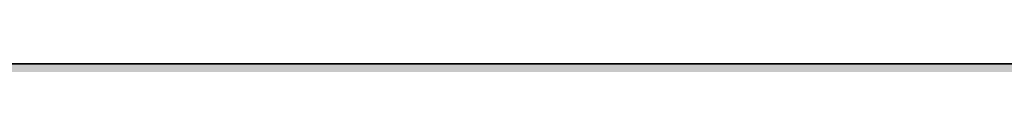
# Model space of a CAD drawing. Units: inches. Extents: x 2091 to 2899, y 967 to 2217.
# Tile 74 of 256: x 2217.572 to 2223.202, y 1099.919 to 1099.919. Entities that reach past the tile are written whole.
import ezdxf

# ---------------------------------------------------------------- set-up
doc = ezdxf.new("R2010")
doc.units = ezdxf.units.IN
doc.layers.add('A-WALL-PATT', color=141, linetype='Continuous', lineweight=13, true_color=0xadddf7)
doc.layers.add('L-SITE-WALL', color=7, linetype='Continuous', lineweight=35)

msp = doc.modelspace()

# ---------------------------------------------------------------- hatches: boundary and pattern name
at = {"layer": 'A-WALL-PATT'}
h = msp.add_hatch(color=256, dxfattribs=at)
h.dxf.hatch_style = 1
h.paths.add_polyline_path([(2212.1436, 1941.4191), (2387.6436, 1941.4191), (2387.6436, 1824.4191), (2392.1436, 1824.4191), (2392.1436, 1941.4191), (2609.6436, 1941.4191), (2609.6436, 1825.9191), (2614.1436, 1825.9191), (2614.1436, 1941.4191), (2794.1436, 1941.4191), (2794.1436, 1928.7622), (2803.1436, 1928.7622), (2803.1436, 2050.9191), (2203.1436, 2050.9191), (2203.1436, 1900.7579), (2212.1436, 1900.7579)])
h.paths.add_polyline_path([(2212.1436, 1945.9191), (2212.1436, 2041.9191), (2794.1436, 2041.9191), (2794.1436, 1945.9191), (2402.2482, 1945.9191), (2401.1024, 1945.7758), (2398.7024, 1945.7758)], flags=16)
h.paths.add_polyline_path([(2230.2299, 1948.0628), (2227.3499, 1949.5028), (2225.9099, 1951.9028), (2223.9899, 1952.8628), (2223.0299, 1955.2628), (2222.0699, 1959.5828), (2222.0699, 1963.4228), (2223.0299, 1965.6628), (2223.9899, 1965.3428), (2225.5859, 1963.8607), (2226.9115, 1964.9573), (2226.9489, 1965.9388), (2227.7783, 1966.9521), (2228.1999, 1968.8787), (2230.7099, 1964.8628), (2233.5899, 1966.3028), (2233.6073, 1966.3319), (2233.7727, 1964.9382), (2234.6338, 1963.6765), (2235.0299, 1963.9028), (2236.282, 1965.5724), (2235.9899, 1962.9428), (2237.9545, 1957.54), (2238.3899, 1957.9028), (2239.2159, 1960.3058), (2238.6546, 1966.385), (2238.6928, 1966.4381), (2238.8406, 1967.4997), (2238.7803, 1967.6875), (2238.8805, 1967.7868), (2238.6669, 1966.2518), (2239.2159, 1960.3058), (2238.3899, 1957.9028), (2236.9499, 1956.7028), (2234.5499, 1949.9828)], flags=0)
h.paths.add_polyline_path([(2278.012, 1948.0628), (2276.4964, 1947.8733), (2275.8498, 1947.6886), (2274.652, 1947.1028)], flags=0)
h.paths.add_polyline_path([(2269.852, 1955.7428), (2268.2762, 1956.6293), (2270.8673, 1956.3484), (2269.372, 1958.1428), (2268.715, 1959.1923), (2270.5698, 1958.7286), (2268.5807, 1961.9061), (2270.812, 1960.8919), (2270.812, 1963.4228), (2271.3933, 1964.7793), (2270.2918, 1966.1562), (2271.772, 1965.6628), (2272.1414, 1966.5248), (2273.9298, 1965.9286), (2275.6304, 1968.0543), (2276.3319, 1966.7219), (2276.5204, 1966.9521), (2276.942, 1968.8787), (2277.7343, 1967.6111), (2278.1399, 1969.4645), (2279.6591, 1967.0337), (2280.412, 1966.7828), (2280.9493, 1967.5888), (2281.6098, 1967.3686), (2282.1333, 1968.1538), (2282.3492, 1966.3334), (2282.3498, 1966.3326), (2283.4076, 1968.0954), (2283.7126, 1965.524), (2284.3202, 1964.6338), (2284.5118, 1964.8892), (2284.235, 1965.7048), (2284.5005, 1967.319), (2284.9079, 1965.4174), (2285.3963, 1966.0686), (2285.4328, 1966.2906), (2285.4733, 1966.1713), (2286.3539, 1967.3454), (2286.222, 1966.1582), (2287.6635, 1968.0802), (2287.714, 1968.4428), (2288.4816, 1969.0167), (2288.574, 1968.7289), (2288.9175, 1969.069), (2288.6068, 1966.8376), (2288.9287, 1963.3513), (2288.935, 1963.3568), (2288.9297, 1963.3404), (2289.0153, 1962.4139), (2290.1112, 1963.8751), (2290.1328, 1963.9426), (2290.2177, 1964.0171), (2290.1112, 1963.8751), (2289.1558, 1960.8916), (2288.594, 1959.2572), (2288.572, 1959.1028), (2289.532, 1960.5428), (2290.012, 1962.4628), (2290.1918, 1962.6427), (2289.7698, 1959.6886), (2286.8898, 1957.2886), (2284.4898, 1950.5686), (2283.3147, 1950.0463), (2283.292, 1949.9828), (2280.2901, 1948.6486), (2281.1298, 1948.6486), (2282.5698, 1948.1686), (2283.2047, 1948.0628), (2278.972, 1948.0628), (2276.092, 1949.5028), (2274.652, 1951.9028), (2272.732, 1952.8628)], flags=0)
h.paths.add_polyline_path([(2271.1589, 1958.0218), (2272.9698, 1955.8486), (2272.0098, 1960.1686), (2272.0098, 1964.0086), (2272.6244, 1965.4427), (2274.328, 1963.8607), (2275.6536, 1964.9573), (2275.6377, 1964.5391), (2277.4122, 1966.0069), (2277.033, 1965.1568), (2276.8299, 1964.9756), (2276.766, 1963.295), (2277.4496, 1962.6602), (2279.452, 1964.8628), (2282.332, 1966.3028), (2283.5298, 1966.8886), (2283.2945, 1966.7709), (2283.913, 1963.8847), (2284.8992, 1964.4483), (2284.732, 1962.9428), (2286.6966, 1957.54), (2287.132, 1957.9028), (2287.5419, 1959.0954), (2287.7794, 1958.4423), (2285.6827, 1956.6951), (2285.8765, 1959.7953), (2284.732, 1962.9428), (2284.8992, 1964.4483), (2283.913, 1963.8847), (2284.2238, 1962.4341), (2283.4244, 1963.6055), (2281.6098, 1962.5686), (2281.1298, 1960.1686), (2282.0898, 1956.3286), (2283.0498, 1952.9686), (2282.5698, 1950.5686), (2280.1698, 1948.6486), (2279.8833, 1948.7919), (2278.972, 1948.0628), (2278.972, 1949.0228), (2278.6723, 1949.3974), (2277.2898, 1950.0886), (2275.8498, 1952.4886), (2273.9298, 1953.4486), (2272.4898, 1954.8886), (2271.9216, 1954.8886), (2271.772, 1955.2628)], flags=0)
h.paths.add_polyline_path([(2311.9941, 1955.7428), (2312.0627, 1955.6742), (2312.0551, 1955.7085)], flags=0)
h.paths.add_polyline_path([(2331.9561, 1963.9518), (2333.3961, 1965.3918), (2331.0771, 1963.3568), (2330.9986, 1963.1115)], flags=0)
h.paths.add_polyline_path([(2310.5541, 1954.3028), (2307.0398, 1956.2799), (2310.7629, 1955.8763), (2312.4741, 1953.8228), (2313.4341, 1951.4228), (2315.3541, 1950.4628), (2316.7941, 1948.0628), (2317.4661, 1947.7268), (2319.3687, 1947.9646), (2317.7541, 1949.9828), (2317.5695, 1950.6105), (2316.7941, 1951.9028), (2314.8741, 1952.8628), (2313.9141, 1955.2628), (2311.5141, 1958.1428), (2309.3755, 1961.5592), (2311.5141, 1960.3371), (2311.5141, 1961.9828), (2310.6047, 1963.1196), (2311.7266, 1962.4785), (2312.4183, 1964.0926), (2312.256, 1964.2955), (2313.1941, 1963.9828), (2313.9141, 1965.6628), (2314.6468, 1965.4186), (2315.3541, 1966.3028), (2316.7941, 1967.7428), (2316.1574, 1966.9469), (2317.0341, 1965.2819), (2317.2226, 1965.5121), (2317.777, 1968.0458), (2318.4741, 1966.7219), (2318.6626, 1966.9521), (2319.0842, 1968.8787), (2321.207, 1965.4821), (2322.1614, 1966.9137), (2322.5541, 1966.7828), (2322.786, 1967.1306), (2322.8816, 1966.3243), (2323.312, 1965.7217), (2323.6513, 1965.8914), (2324.3965, 1967.1334), (2324.6569, 1964.9382), (2324.972, 1964.4766), (2325.3873, 1967.0015), (2325.9408, 1964.4183), (2327.2289, 1966.1358), (2327.1663, 1965.5724), (2328.0591, 1966.7628), (2328.2246, 1966.2475), (2329.668, 1967.6769), (2329.6646, 1967.6875), (2329.7648, 1967.7868), (2329.5511, 1966.2518), (2330.1001, 1960.3058), (2329.3328, 1958.0735), (2329.3131, 1957.9352), (2329.6341, 1958.2028), (2330.2341, 1959.1028), (2330.7141, 1961.0228), (2331.0341, 1961.3428), (2330.7141, 1959.1028), (2329.6341, 1958.2028), (2329.2741, 1957.6628), (2327.7121, 1956.3611), (2325.4341, 1949.9828), (2324.3338, 1949.4937), (2323.9941, 1948.5428), (2319.6741, 1946.6228), (2316.7941, 1948.0628), (2315.3541, 1950.4628), (2313.4341, 1951.4228)], flags=0)
h.paths.add_polyline_path([(2321.3357, 1947.952), (2321.1141, 1948.0628), (2321.1141, 1949.0228), (2319.1941, 1951.4228), (2316.7941, 1959.5828), (2316.6632, 1959.5828), (2315.3541, 1958.1428), (2314.3941, 1958.1428), (2313.1483, 1958.7091), (2312.9541, 1959.5828), (2312.9541, 1960.8919), (2315.8341, 1959.5828), (2316.6632, 1959.5828), (2317.3147, 1960.2994), (2315.0302, 1962.4207), (2316.3558, 1963.5173), (2316.3723, 1963.9516), (2316.4702, 1963.8607), (2317.7958, 1964.9573), (2317.7552, 1963.8897), (2319.1751, 1965.1568), (2319.4984, 1965.8814), (2321.1141, 1965.3428), (2323.2359, 1962.3724), (2325.6863, 1963.7726), (2325.5428, 1962.4806), (2325.1988, 1963.494), (2324.4785, 1963.0824), (2324.926, 1960.9941), (2324.0781, 1962.2365), (2322.4148, 1961.286), (2322.0741, 1959.5828), (2323.0341, 1955.7428), (2323.9941, 1952.3828), (2323.5141, 1949.9828), (2322.1427, 1948.8856), (2322.0741, 1948.5428)], flags=0)
h.paths.add_polyline_path([(2320.2075, 1963.3375), (2320.1541, 1963.4228), (2320.3941, 1963.5428)], flags=0)
h.paths.add_polyline_path([(2353.8505, 1965.8105), (2354.0305, 1965.7505), (2354.3305, 1966.4505), (2354.3305, 1966.9305)], flags=0)
h.paths.add_polyline_path([(2359.0206, 1969.0264), (2359.0984, 1968.9019), (2359.2335, 1969.5195), (2359.2335, 1969.9995)], flags=0)
h.paths.add_polyline_path([(2358.2567, 1966.6817), (2357.9836, 1966.348), (2358.2113, 1966.1462), (2358.4105, 1966.3896)], flags=0)
h.paths.add_polyline_path([(2357.7685, 1966.0588), (2357.7322, 1965.105), (2357.751, 1965.1206), (2357.7695, 1965.6065), (2357.7695, 1966.0578)], flags=0)
h.paths.add_polyline_path([(2359.1115, 1965.3045), (2359.1115, 1964.8245), (2359.8445, 1966.4675), (2359.8445, 1966.9475)], flags=0)
h.paths.add_polyline_path([(2360.2237, 1966.6214), (2360.6985, 1969.3625), (2360.6985, 1969.8425), (2360.2105, 1967.0255), (2360.2105, 1966.6425)], flags=0)
h.paths.add_polyline_path([(2363.4505, 1967.8905), (2363.4505, 1968.3705), (2362.4905, 1966.9305), (2362.656, 1966.6988)], flags=0)
h.paths.add_polyline_path([(2364.4755, 1966.0788), (2365.8505, 1968.3705), (2365.8505, 1968.8505), (2364.428, 1966.4796)], flags=0)
h.paths.add_polyline_path([(2366.3135, 1965.8525), (2366.3667, 1965.6958), (2366.8025, 1968.3455), (2366.8025, 1968.8255)], flags=0)
h.paths.add_polyline_path([(2367.1653, 1965.8035), (2367.2905, 1966.9305), (2367.2905, 1967.4105), (2367.1027, 1965.7201)], flags=0)
h.paths.add_polyline_path([(2370.0365, 1959.9735), (2371.0135, 1963.0245), (2371.0135, 1963.5045), (2370.0365, 1960.4535)], flags=0)
h.paths.add_polyline_path([(2371.6105, 1960.2105), (2372.5705, 1961.6505), (2372.5705, 1962.1305), (2371.8025, 1960.9785)], flags=0)
h.paths.add_polyline_path([(2350.8737, 1956.0051), (2351.9305, 1955.8905), (2354.4905, 1953.3305), (2353.8505, 1954.9305), (2351.4505, 1957.8105), (2347.9355, 1963.4255), (2347.9355, 1963.9055), (2351.4505, 1958.2905), (2353.7051, 1955.585), (2352.8905, 1959.2505), (2352.8905, 1959.7305), (2352.8905, 1961.9248), (2356.7305, 1959.7305), (2358.4545, 1961.6268), (2354.8105, 1965.0105), (2355.0309, 1965.2859), (2358.6911, 1961.8871), (2361.5305, 1965.0105), (2364.3765, 1966.4335), (2364.5244, 1965.1869), (2365.4545, 1963.8242), (2365.8811, 1964.068), (2365.3705, 1966.4505), (2365.3705, 1966.9305), (2366.8105, 1960.2105), (2366.8105, 1959.7305), (2366.3887, 1952.9814), (2367.7705, 1956.8505), (2368.6412, 1957.5761), (2366.8105, 1962.6105), (2366.8105, 1963.0905), (2368.7752, 1957.6877), (2369.2105, 1958.0505), (2370.0016, 1960.3519), (2369.4752, 1966.0527), (2369.5135, 1966.1058), (2369.5142, 1966.1109), (2369.4752, 1966.5327), (2369.5135, 1966.5858), (2369.6146, 1967.3126), (2369.1825, 1968.6585), (2369.1825, 1969.1385), (2369.601, 1967.8352), (2369.7012, 1967.9345), (2369.7179, 1968.0547), (2370.1452, 1968.3741), (2369.7787, 1968.0112), (2369.7012, 1967.4545), (2370.4682, 1968.214), (2369.6749, 1967.2658), (2369.5142, 1966.1109), (2370.0365, 1960.4535), (2370.0365, 1959.9735), (2369.4418, 1958.2432), (2370.6505, 1959.2505), (2371.0458, 1962.0176), (2371.1305, 1962.1305), (2370.6505, 1958.7705), (2367.7705, 1956.3705), (2365.3705, 1949.6505), (2362.0791, 1948.1876), (2363.4505, 1947.7305), (2361.0505, 1947.7305), (2360.0905, 1947.7305), (2357.1039, 1947.3572), (2360.0905, 1948.2105), (2358.1705, 1949.1705), (2356.7305, 1951.5705), (2354.8105, 1952.5305), (2351.9305, 1955.4105)], flags=0)
h.paths.add_polyline_path([(2361.0505, 1948.6905), (2359.1305, 1951.0905), (2356.7305, 1959.2505), (2355.7705, 1959.2505), (2352.8905, 1960.5596), (2352.8905, 1961.4448), (2355.8905, 1959.7305), (2356.7305, 1959.7305), (2356.8372, 1959.3678), (2361.5305, 1964.5305), (2363.2484, 1965.3894), (2364.9253, 1963.0418), (2362.4905, 1961.6505), (2362.0639, 1959.5172), (2362.9705, 1955.8905), (2363.9305, 1952.5305), (2363.9305, 1952.0505), (2363.4505, 1949.6505), (2361.0505, 1947.7305)], flags=0)
h.paths.add_polyline_path([(2359.1305, 1951.5705), (2359.2905, 1951.3705), (2361.0505, 1954.4505), (2361.0505, 1954.9305)], flags=0)
h.paths.add_polyline_path([(2357.2195, 1966.5455), (2356.7925, 1968.8145), (2356.7925, 1969.2945), (2357.2195, 1967.0255)], flags=0)
h.paths.add_polyline_path([(2361.0505, 1954.4505), (2361.5305, 1958.7705), (2361.5305, 1959.2505), (2361.0505, 1954.9305)], flags=0)
h.paths.add_polyline_path([(2402.5483, 1948.4861), (2402.3024, 1948.4158), (2402.5904, 1948.4158)], flags=0)
h.paths.add_polyline_path([(2394.1424, 1956.0958), (2395.6851, 1954.5532), (2396.7205, 1953.9707), (2396.0624, 1955.6158), (2395.2414, 1956.6011), (2395.8789, 1956.4417), (2395.1024, 1959.9358), (2395.1024, 1963.7758), (2396.0624, 1966.0158), (2397.0224, 1965.6958), (2398.6185, 1964.2138), (2399.9441, 1965.3103), (2399.9814, 1966.2918), (2400.8109, 1967.3052), (2401.2325, 1969.2317), (2403.5379, 1965.543), (2403.942, 1967.3893), (2404.7024, 1967.1358), (2405.4603, 1966.0748), (2406.6224, 1966.6558), (2406.6399, 1966.6849), (2406.8052, 1965.2912), (2406.9257, 1965.1147), (2407.3424, 1964.9758), (2407.8743, 1965.7737), (2408.1691, 1964.3981), (2409.3146, 1965.9254), (2409.2175, 1965.0511), (2409.4452, 1963.1312), (2410.3064, 1961.8695), (2410.7024, 1962.0958), (2411.4423, 1963.0823), (2411.1654, 1963.8978), (2411.6164, 1966.6398), (2411.7254, 1966.7911), (2411.8732, 1967.8527), (2411.8129, 1968.0405), (2411.9131, 1968.1398), (2411.6994, 1966.6048), (2412.2484, 1960.6588), (2413.2254, 1963.7098), (2414.3779, 1964.7212), (2414.5132, 1965.6927), (2414.4529, 1965.8805), (2414.5531, 1965.9798), (2414.3779, 1964.7212), (2414.5198, 1964.8457), (2414.3654, 1964.6311), (2414.3394, 1964.4448), (2414.8884, 1958.4988), (2414.0624, 1956.0958), (2412.6224, 1954.8958), (2410.1714, 1948.0329), (2410.0167, 1948.0844), (2405.9024, 1946.2558), (2405.9024, 1947.2158), (2405.2043, 1948.0886), (2404.2224, 1948.4158), (2403.2624, 1948.4158), (2400.3824, 1949.8558), (2399.6624, 1951.0558), (2397.9824, 1952.7358), (2397.0224, 1953.2158), (2395.6851, 1954.5532), (2392.6568, 1956.2569)], flags=0)
h.paths.add_polyline_path([(2409.0857, 1964.4074), (2409.1304, 1964.2757), (2409.2624, 1964.4958)], flags=0)
h.paths.add_polyline_path([(2397.7424, 1961.6158), (2398.7024, 1963.8558), (2399.6624, 1963.5358), (2401.4266, 1965.741), (2401.7914, 1966.5588), (2402.0714, 1965.0708), (2402.8355, 1964.3934), (2403.2624, 1964.9149), (2403.3381, 1964.7711), (2402.6155, 1963.9762), (2402.4986, 1960.9022), (2403.543, 1959.9325), (2404.4132, 1960.8897), (2404.7024, 1962.3358), (2407.9163, 1964.1724), (2409.5202, 1961.9269), (2410.9871, 1957.893), (2411.4224, 1958.2558), (2412.048, 1960.0756), (2412.4103, 1959.0791), (2411.6756, 1958.4668), (2411.6624, 1958.2558), (2411.6261, 1958.4255), (2409.9824, 1957.0558), (2407.5824, 1950.3358), (2403.2624, 1948.4158), (2403.2624, 1949.3758), (2401.3424, 1951.7758), (2399.4165, 1958.324), (2397.7424, 1959.0849), (2397.7424, 1959.9701), (2397.1024, 1960.3358), (2397.7424, 1960.0449)], flags=0)
h.paths.add_polyline_path([(2405.9024, 1952.9758), (2405.9504, 1953.4078), (2406.0167, 1953.1758)], flags=0)
h.paths.add_polyline_path([(2449.8178, 1967.114), (2449.7523, 1967.1358), (2449.7937, 1967.0779)], flags=0)
h.paths.add_polyline_path([(2451.6977, 1966.6181), (2451.7409, 1966.6901), (2451.6921, 1966.6657)], flags=0)
h.paths.add_polyline_path([(2454.3436, 1965.7376), (2455.7523, 1967.6158), (2455.9923, 1968.0958), (2454.3645, 1965.9254)], flags=0)
h.paths.add_polyline_path([(2457.5473, 1968.8638), (2457.7873, 1969.3438), (2457.0543, 1968.7958), (2457.0076, 1968.4603)], flags=0)
h.paths.add_polyline_path([(2456.9218, 1967.8567), (2456.8022, 1968.229), (2456.723, 1967.6598)], flags=0)
h.paths.add_polyline_path([(2457.3023, 1967.3768), (2457.5423, 1967.8568), (2456.8103, 1966.8398), (2456.7405, 1966.7002), (2456.749, 1966.6081)], flags=0)
h.paths.add_polyline_path([(2458.2753, 1963.7098), (2458.1553, 1963.3352), (2460.3543, 1965.2648), (2460.5943, 1965.7448)], flags=0)
h.paths.add_polyline_path([(2458.3923, 1962.8158), (2458.3641, 1962.6182), (2459.5923, 1964.2558), (2459.8323, 1964.7358)], flags=0)
h.paths.add_polyline_path([(2459.3523, 1962.8158), (2459.2723, 1962.4958), (2460.0723, 1963.2958), (2460.3123, 1963.7758)], flags=0)
h.paths.add_polyline_path([(2458.6803, 1960.6078), (2458.6323, 1960.4158), (2459.5923, 1961.8558), (2459.8323, 1962.3358)], flags=0)
h.paths.add_polyline_path([(2437.8382, 1956.2427), (2439.1923, 1956.0958), (2441.3523, 1953.9358), (2440.8723, 1955.1358), (2438.4723, 1958.0158), (2438.0716, 1958.656), (2438.7123, 1958.4958), (2440.6396, 1956.1831), (2439.9123, 1959.4558), (2439.9123, 1963.2958), (2441.3523, 1966.6558), (2441.5923, 1967.1358), (2441.1123, 1966.0158), (2442.0723, 1965.6958), (2443.989, 1968.0917), (2444.2413, 1966.7508), (2444.9168, 1966.1519), (2445.6766, 1967.0801), (2446.2553, 1969.7248), (2446.4953, 1970.2048), (2446.2824, 1969.2317), (2447.3627, 1967.5033), (2447.7203, 1969.5678), (2447.9603, 1970.0478), (2447.4855, 1967.3068), (2448.7923, 1965.2158), (2448.4723, 1964.8638), (2448.5523, 1964.7358), (2451.4521, 1966.1857), (2451.6151, 1964.8112), (2452.3079, 1963.7962), (2453.2345, 1964.3257), (2454.0723, 1960.4158), (2453.6287, 1953.3177), (2454.7923, 1956.5758), (2455.0323, 1957.0558), (2455.7188, 1957.6279), (2453.8323, 1962.8158), (2453.941, 1963.7936), (2453.3353, 1965.5778), (2453.8243, 1968.5508), (2454.0643, 1969.0308), (2453.5753, 1966.0578), (2454.0403, 1964.6879), (2453.8323, 1962.8158), (2455.7188, 1957.6279), (2456.3672, 1958.1682), (2457.0583, 1960.1788), (2457.2983, 1960.6588), (2456.4723, 1958.2558), (2457.7177, 1959.2937), (2457.6723, 1958.9758), (2454.89, 1956.6572), (2453.6141, 1953.0849), (2453.5923, 1952.7358), (2453.3523, 1952.2558), (2453.3596, 1952.3722), (2452.6323, 1950.3358), (2452.3923, 1949.8558), (2449.2038, 1948.4387), (2450.7123, 1947.9358), (2448.0723, 1947.9358), (2447.1123, 1947.9358), (2444.5523, 1947.6158), (2447.1996, 1948.3722), (2445.1923, 1949.3758), (2443.7523, 1951.7758), (2441.8323, 1952.7358), (2438.9523, 1955.6158)], flags=0)
h.paths.add_polyline_path([(2443.9923, 1959.9358), (2444.0403, 1959.7726), (2444.1216, 1959.862)], flags=0)
h.paths.add_polyline_path([(2442.9123, 1959.9358), (2443.0323, 1959.9358), (2442.4457, 1960.2025)], flags=0)
h.paths.add_polyline_path([(2444.9829, 1965.0197), (2445.2793, 1965.2648), (2445.5193, 1965.7448), (2444.994, 1965.3103)], flags=0)
h.paths.add_polyline_path([(2446.1333, 1965.0298), (2446.3304, 1965.4715), (2444.9703, 1964.2578), (2444.7303, 1963.7778)], flags=0)
h.paths.add_polyline_path([(2442.7923, 1959.4558), (2443.7523, 1959.4558), (2446.1523, 1951.2958), (2446.4123, 1951.7508), (2446.3923, 1951.7758), (2448.0806, 1954.7303), (2448.5523, 1958.9758), (2441.8323, 1965.2158), (2442.1549, 1965.6191), (2448.7923, 1959.4558), (2448.3123, 1955.1358), (2448.0723, 1954.6558), (2446.4123, 1951.7508), (2448.3123, 1949.3758), (2448.3123, 1948.4158), (2450.5409, 1950.1987), (2450.9523, 1952.2558), (2449.9923, 1955.6158), (2449.0323, 1959.4558), (2449.5123, 1961.8558), (2449.7523, 1962.3358), (2449.6749, 1961.9487), (2452.9945, 1963.8457), (2453.0644, 1963.5194), (2452.8846, 1963.7829), (2449.6749, 1961.9487), (2449.2723, 1959.9358), (2450.2323, 1956.0958), (2451.1923, 1952.7358), (2450.7123, 1950.3358), (2450.4723, 1949.8558), (2448.0723, 1947.9358), (2448.0723, 1948.5358), (2445.4323, 1949.8558), (2443.9923, 1952.2558), (2442.0723, 1953.2158), (2441.1123, 1955.6158), (2440.1523, 1959.9358), (2440.1523, 1960.6558)], flags=0)
h.paths.add_polyline_path([(2456.6923, 1966.9858), (2457.6083, 1968.0808), (2457.8483, 1968.5608), (2456.9323, 1967.4658)], flags=0)
h.paths.add_polyline_path([(2489.8966, 1966.5802), (2489.9429, 1966.1893), (2490.7475, 1967.5302), (2491.3191, 1968.9512)], flags=0)
h.paths.add_polyline_path([(2473.5625, 1956.4071), (2477.14, 1956.0193), (2476.9553, 1956.2408), (2475.108, 1957.2801), (2476.3475, 1956.9702), (2475.1869, 1958.8242), (2476.9191, 1958.3912), (2475.4116, 1960.7993), (2477.7875, 1959.7193), (2477.7875, 1962.2502), (2477.6374, 1962.4379), (2477.8226, 1962.3321), (2478.3591, 1963.5841), (2478.3591, 1963.6712), (2477.3243, 1964.9646), (2478.7148, 1964.5011), (2479.3191, 1965.9112), (2480.2791, 1965.5912), (2481.784, 1967.4722), (2482.1165, 1965.7052), (2482.8806, 1965.0278), (2483.2093, 1965.4294), (2483.2202, 1965.7151), (2483.0759, 1965.989), (2483.7118, 1966.7658), (2484.1305, 1968.6792), (2484.7021, 1970.1002), (2484.4892, 1969.1271), (2486.5029, 1965.9051), (2487.3875, 1965.6102), (2488.1534, 1966.7591), (2488.717, 1965.9701), (2489.2001, 1966.2116), (2489.3307, 1965.111), (2490.3939, 1963.6225), (2490.6608, 1963.775), (2490.4939, 1964.5536), (2490.9231, 1963.9248), (2491.3191, 1964.1512), (2491.3334, 1964.1702), (2491.2105, 1964.5322), (2491.2818, 1964.9655), (2491.4258, 1964.2934), (2494.0765, 1967.8276), (2494.4979, 1966.5149), (2494.5982, 1966.6142), (2494.6895, 1967.2702), (2495.1067, 1967.5822), (2495.1298, 1967.7481), (2495.0696, 1967.9359), (2495.1698, 1968.0351), (2495.0318, 1967.0436), (2495.7538, 1967.7587), (2494.9821, 1966.6864), (2494.9561, 1966.5002), (2495.479, 1960.8369), (2495.9105, 1962.1842), (2496.4821, 1963.6052), (2496.0727, 1962.3266), (2496.7689, 1962.9375), (2496.5991, 1962.7112), (2496.1191, 1959.3512), (2496.7329, 1960.2718), (2496.9875, 1961.2902), (2497.5591, 1962.7112), (2497.0791, 1960.7912), (2496.5075, 1959.3702), (2495.5475, 1957.9302), (2492.7588, 1955.6064), (2490.8391, 1950.2312), (2490.2675, 1948.8102), (2485.9475, 1946.8902), (2483.0675, 1948.3302), (2481.6275, 1950.7302), (2479.7075, 1951.6902), (2476.8275, 1954.5702)], flags=0)
h.paths.add_polyline_path([(2485.577, 1948.3134), (2485.5591, 1948.3112), (2485.5788, 1948.3112)], flags=0)
h.paths.add_polyline_path([(2478.6451, 1954.5512), (2478.109, 1956.9633), (2479.3191, 1955.5112), (2480.2791, 1953.1112), (2482.1991, 1952.1512), (2483.6391, 1949.7512), (2486.5191, 1948.3112), (2486.5191, 1949.2712), (2484.7393, 1951.4959), (2484.0275, 1950.2502), (2481.6275, 1958.4102), (2482.3751, 1959.2327), (2482.1991, 1959.8312), (2483.1976, 1960.9295), (2479.7075, 1964.1702), (2480.6034, 1965.2901), (2481.8752, 1964.1091), (2482.6664, 1964.7636), (2482.6154, 1963.4218), (2482.9892, 1963.0747), (2484.0085, 1963.9842), (2484.6836, 1965.4975), (2484.5801, 1965.4052), (2485.3573, 1967.1471), (2485.1206, 1965.7812), (2486.4275, 1963.6902), (2488.1454, 1964.5492), (2489.8223, 1962.2016), (2490.7475, 1962.7302), (2491.9997, 1964.3998), (2492.076, 1965.0873), (2492.2129, 1964.6841), (2492.4854, 1965.0474), (2492.2791, 1963.1912), (2494.2438, 1957.7884), (2494.5625, 1958.054), (2494.9335, 1959.1332), (2495.5051, 1960.5542), (2494.6791, 1958.1512), (2494.1075, 1956.7302), (2494.5625, 1958.054), (2493.4085, 1957.0923), (2491.7075, 1961.7702), (2491.9997, 1964.3998), (2490.7475, 1962.7302), (2487.712, 1960.9957), (2487.4791, 1959.8312), (2488.4391, 1955.9912), (2489.3991, 1952.6312), (2488.9191, 1950.2312), (2488.5769, 1949.9574), (2488.3475, 1948.8102), (2487.6517, 1948.2536), (2487.4791, 1948.3112), (2486.5191, 1948.3112), (2483.6391, 1949.7512), (2482.1991, 1952.1512), (2480.2791, 1953.1112), (2478.8391, 1954.5512)], flags=0)
h.paths.add_polyline_path([(2526.6483, 1966.9875), (2526.5173, 1967.0312), (2526.6001, 1966.9153)], flags=0)
h.paths.add_polyline_path([(2528.4706, 1966.4467), (2528.5745, 1966.6197), (2528.4571, 1966.561)], flags=0)
h.paths.add_polyline_path([(2534.1333, 1967.4962), (2534.1567, 1967.5428), (2534.0598, 1967.4083)], flags=0)
h.paths.add_polyline_path([(2536.1619, 1964.0506), (2535.1573, 1962.7112), (2535.1009, 1962.3159), (2536.1173, 1963.6712), (2536.4205, 1964.2775)], flags=0)
h.paths.add_polyline_path([(2535.1573, 1959.8312), (2536.1173, 1961.2712), (2536.5973, 1962.2312), (2535.2533, 1960.2152)], flags=0)
h.paths.add_polyline_path([(2513.249, 1956.2848), (2516.2212, 1955.9626), (2514.9973, 1957.4312), (2514.1958, 1958.7115), (2515.4773, 1958.3912), (2516.9319, 1956.6457), (2516.4373, 1958.8712), (2516.4373, 1962.7112), (2516.8727, 1963.727), (2515.3464, 1965.6348), (2517.3973, 1964.9512), (2517.8773, 1966.0712), (2518.3573, 1967.0312), (2517.8773, 1965.9112), (2518.8373, 1965.5912), (2520.4866, 1967.6527), (2520.7663, 1966.1662), (2521.5304, 1965.4887), (2521.7814, 1965.7954), (2521.8009, 1966.3073), (2521.4778, 1966.9209), (2521.2463, 1967.1262), (2521.1777, 1967.4909), (2521.4778, 1966.9209), (2522.0104, 1966.4487), (2522.2574, 1966.7504), (2522.7803, 1969.1402), (2523.2603, 1970.1002), (2523.0474, 1969.1271), (2524.6731, 1966.5259), (2526.0373, 1966.0712), (2526.7952, 1965.0101), (2527.9771, 1965.601), (2528.1401, 1964.2266), (2528.6646, 1963.4582), (2529.3886, 1963.8719), (2529.3297, 1964.147), (2529.4813, 1963.9248), (2529.8773, 1964.1512), (2529.984, 1964.2934), (2529.7891, 1965.2032), (2530.0624, 1964.3979), (2532.8025, 1968.0513), (2533.1478, 1966.9759), (2533.248, 1967.0751), (2533.3393, 1967.7312), (2533.6728, 1967.9805), (2533.728, 1968.0351), (2533.5143, 1966.5002), (2534.0247, 1960.9725), (2534.5603, 1962.6452), (2535.0403, 1963.6052), (2534.0633, 1960.5542), (2533.2373, 1958.1512), (2534.2882, 1959.0268), (2534.1973, 1958.3912), (2531.5126, 1956.1539), (2529.3973, 1950.2312), (2528.9173, 1949.2712), (2526.4488, 1948.174), (2527.4773, 1947.8312), (2530.3573, 1947.3512), (2524.5973, 1947.3512), (2521.7173, 1948.7912), (2520.2773, 1951.1912), (2518.3573, 1952.1512), (2515.4773, 1955.0312)], flags=0)
h.paths.add_polyline_path([(2523.9348, 1967.1903), (2523.6195, 1966.4837), (2523.7705, 1966.2421)], flags=0)
h.paths.add_polyline_path([(2518.8373, 1953.1112), (2517.8773, 1955.5112), (2516.885, 1959.9768), (2516.9173, 1959.9621), (2516.9173, 1962.0254), (2520.7573, 1959.8312), (2522.0249, 1961.2255), (2518.3573, 1964.6312), (2519.0026, 1965.4377), (2520.4334, 1964.1091), (2521.3011, 1964.8269), (2521.2452, 1963.3553), (2525.6383, 1959.276), (2526.0373, 1961.2712), (2529.3973, 1963.1912), (2530.6495, 1964.8607), (2530.6647, 1964.9976), (2530.692, 1964.9173), (2531.0878, 1965.4451), (2530.946, 1964.1689), (2530.692, 1964.9173), (2529.3973, 1963.1912), (2526.3625, 1961.457), (2526.0373, 1959.8312), (2526.9973, 1955.9912), (2527.9573, 1952.6312), (2527.4773, 1950.2312), (2527.1345, 1949.9569), (2526.9739, 1949.1541), (2526.6973, 1949.0312), (2524.5973, 1947.3512), (2524.5973, 1948.3112), (2524.2773, 1948.7112), (2522.1973, 1949.7512), (2520.7573, 1952.1512)], flags=0)
h.paths.add_polyline_path([(2520.2773, 1958.8712), (2520.8533, 1959.5048), (2523.1573, 1951.6712), (2524.6139, 1954.2201), (2524.5973, 1954.0712), (2522.6773, 1950.7112)], flags=0)
h.paths.add_polyline_path([(2559.3709, 1966.3112), (2559.3984, 1966.3249), (2559.4019, 1966.3453)], flags=0)
h.paths.add_polyline_path([(2549.7709, 1957.1912), (2552.6509, 1954.3112), (2552.134, 1955.6035), (2550.6109, 1957.4312), (2547.0959, 1963.0462), (2545.7759, 1965.2062), (2549.2909, 1959.5912), (2551.6909, 1956.7112), (2550.7929, 1960.7521), (2550.7309, 1960.7803), (2550.7309, 1964.8712), (2551.6909, 1967.1112), (2552.6509, 1966.7912), (2554.247, 1965.3091), (2555.0343, 1965.9603), (2555.5817, 1966.6446), (2555.6099, 1967.3872), (2556.4394, 1968.4005), (2556.861, 1970.3271), (2559.3709, 1966.3112), (2560.6909, 1964.1512), (2562.4088, 1965.0101), (2561.6509, 1966.0712), (2560.3309, 1968.2312), (2561.7585, 1966.2325), (2562.3472, 1967.1156), (2562.4337, 1966.3866), (2563.1278, 1965.3696), (2563.5709, 1965.5912), (2563.5884, 1965.6202), (2563.3625, 1967.5235), (2563.7225, 1965.8438), (2565.06, 1968.073), (2564.7329, 1965.1287), (2565.1176, 1963.3334), (2567.4446, 1966.4361), (2567.3156, 1967.8333), (2567.3538, 1967.8864), (2567.5016, 1968.9481), (2567.4413, 1969.1359), (2567.5416, 1969.2351), (2567.3279, 1967.7002), (2567.8769, 1961.7542), (2568.7467, 1964.4703), (2568.6356, 1965.6733), (2568.6738, 1965.7264), (2568.8216, 1966.7881), (2568.7613, 1966.9759), (2568.8616, 1967.0751), (2568.6479, 1965.5402), (2568.7261, 1964.693), (2568.8539, 1964.8052), (2568.7467, 1964.4703), (2568.8172, 1963.7063), (2568.9709, 1963.9112), (2568.8661, 1963.1773), (2569.1969, 1959.5942), (2568.3709, 1957.1912), (2566.9309, 1955.9912), (2564.6203, 1949.5214), (2564.6509, 1949.5112), (2564.6166, 1949.5112), (2564.5309, 1949.2712), (2560.2109, 1947.3512), (2557.3309, 1948.7912), (2556.0452, 1950.934), (2556.0109, 1950.9512), (2555.8566, 1951.2083), (2553.9709, 1952.1512), (2551.0909, 1955.0312), (2546.6501, 1957.5295)], flags=0)
h.paths.add_polyline_path([(2567.0258, 1959.3302), (2567.035, 1959.3049), (2567.0509, 1959.3512)], flags=0)
h.paths.add_polyline_path([(2551.9683, 1962.5184), (2553.0109, 1964.9512), (2553.9709, 1964.6312), (2555.567, 1963.1491), (2556.8926, 1964.2456), (2556.9299, 1965.2272), (2557.144, 1965.4887), (2556.4201, 1966.1306), (2556.3914, 1966.105), (2556.3799, 1966.1662), (2556.4201, 1966.1306), (2556.9519, 1966.6052), (2557.0921, 1966.9195), (2557.5709, 1966.0102), (2557.7594, 1966.2405), (2557.4179, 1964.6802), (2556.8926, 1964.2456), (2556.8071, 1961.9976), (2560.6909, 1958.3912), (2560.6355, 1957.8927), (2560.8109, 1957.1912), (2561.7709, 1953.8312), (2561.2909, 1951.4312), (2559.1104, 1949.6868), (2559.1565, 1949.6292), (2563.0265, 1951.3492), (2562.6109, 1949.2712), (2560.2109, 1947.3512), (2560.2109, 1948.3112), (2559.2509, 1949.5112), (2558.8909, 1949.5112), (2558.8909, 1949.9612), (2558.2909, 1950.7112), (2558.0537, 1951.5177), (2556.9709, 1952.8712), (2555.0679, 1959.3415), (2552.0509, 1961.0654), (2552.0509, 1962.4712)], flags=0)
h.paths.add_polyline_path([(2588.33, 1958.3912), (2588.6102, 1958.111), (2588.5534, 1958.3669)], flags=0)
h.paths.add_polyline_path([(2594.7455, 1950.4931), (2593.9575, 1953.172), (2593.13, 1954.5512), (2591.21, 1955.5112), (2590.25, 1957.9112), (2588.309, 1960.2404), (2586.1773, 1961.2093), (2587.85, 1960.7912), (2587.2534, 1961.7442), (2588.4413, 1961.0654), (2588.4413, 1962.6555), (2588.4217, 1962.6653), (2588.4413, 1962.7112), (2586.914, 1964.6203), (2588.8771, 1963.728), (2589.29, 1964.6915), (2589.29, 1966.0712), (2590.25, 1968.3112), (2591.21, 1967.9912), (2592.8061, 1966.5091), (2594.1317, 1967.6056), (2594.169, 1968.5872), (2594.9985, 1969.6005), (2595.4201, 1971.5271), (2597.93, 1967.5112), (2600.81, 1968.9512), (2600.8275, 1968.9802), (2600.9928, 1967.5866), (2601.854, 1966.3248), (2602.1071, 1966.4695), (2602.2364, 1967.2551), (2602.3567, 1966.6934), (2603.5022, 1968.2207), (2603.21, 1965.5912), (2605.1747, 1960.1884), (2605.5069, 1960.4652), (2605.026, 1965.6733), (2605.0642, 1965.7264), (2605.212, 1966.7881), (2605.1517, 1966.9759), (2605.252, 1967.0751), (2605.3433, 1967.7312), (2605.9529, 1968.1869), (2605.8748, 1969.0333), (2605.913, 1969.0864), (2606.0608, 1970.1481), (2606.0005, 1970.3359), (2606.1007, 1970.4351), (2605.887, 1968.9002), (2606.436, 1962.9542), (2605.61, 1960.5512), (2605.997, 1960.8737), (2606.5643, 1962.6452), (2608.2415, 1964.1169), (2608.01, 1963.1912), (2607.05, 1961.7512), (2606.6315, 1961.4024), (2606.2013, 1958.3912), (2603.3213, 1955.9912), (2600.9213, 1949.2712), (2596.6013, 1947.3512), (2593.7213, 1948.7912), (2592.8573, 1950.2312), (2592.65, 1950.2312)], flags=0)
h.paths.add_polyline_path([(2596.6013, 1947.3512), (2596.6013, 1948.3112), (2594.6813, 1950.7112), (2596.155, 1953.29), (2595.53, 1954.0712), (2593.1992, 1961.996), (2592.6513, 1962.5047), (2591.7802, 1963.0025), (2593.283, 1964.2456), (2593.3203, 1965.2272), (2594.1498, 1966.2405), (2594.5714, 1968.1671), (2596.1827, 1965.589), (2596.9513, 1966.4345), (2598.0413, 1966.0712), (2598.7992, 1965.0101), (2599.9613, 1965.5912), (2599.9788, 1965.6202), (2600.1441, 1964.2266), (2601.0053, 1962.9648), (2601.4013, 1963.1912), (2602.6535, 1964.8607), (2602.3613, 1962.2312), (2603.7927, 1958.2947), (2601.9776, 1953.2124), (2601.9462, 1952.7095), (2599.4688, 1951.6084), (2599.0013, 1949.2712)], flags=0)
h.paths.add_polyline_path([(2597.5613, 1958.8712), (2597.671, 1959.4194), (2597.5951, 1958.7362)], flags=0)
h.paths.add_polyline_path([(2623.6663, 1961.2544), (2625.5192, 1960.7912), (2624.9655, 1961.6755), (2627.1992, 1960.6603), (2627.1992, 1961.1512), (2626.9592, 1962.2312), (2626.9592, 1963.4912), (2625.5823, 1965.2122), (2626.9592, 1964.4254), (2626.9592, 1965.8312), (2626.8692, 1965.8612), (2627.9192, 1968.3112), (2628.8792, 1967.9912), (2630.4752, 1966.5091), (2631.8008, 1967.6056), (2631.8382, 1968.5872), (2632.6676, 1969.6005), (2633.0892, 1971.5271), (2635.5992, 1967.5112), (2638.4792, 1968.9512), (2638.4966, 1968.9802), (2638.662, 1967.5866), (2639.1763, 1966.833), (2639.7802, 1967.8396), (2640.0258, 1966.6934), (2641.1713, 1968.2207), (2640.8792, 1965.5912), (2641.1143, 1964.9446), (2641.4113, 1965.3407), (2641.3081, 1964.4116), (2642.8438, 1960.1884), (2643.2792, 1960.5512), (2644.0847, 1962.8947), (2643.7839, 1966.1533), (2643.8068, 1966.1852), (2643.6007, 1968.4181), (2643.5228, 1968.6606), (2643.7299, 1970.1481), (2643.6696, 1970.3359), (2643.7698, 1970.4351), (2643.5562, 1968.9002), (2643.6007, 1968.4181), (2643.9096, 1967.4559), (2644.0098, 1967.5551), (2643.8117, 1966.1321), (2644.1052, 1962.9542), (2644.2388, 1961.3508), (2644.7192, 1961.7512), (2645.0329, 1962.2217), (2645.3222, 1963.1252), (2646.0764, 1963.787), (2645.0329, 1962.2217), (2644.3452, 1960.0742), (2643.5192, 1957.6712), (2642.0792, 1956.4712), (2639.7196, 1949.8644), (2639.8755, 1949.8384), (2635.3592, 1947.8312), (2632.4792, 1949.2712), (2631.0392, 1951.6712), (2629.1192, 1952.6312), (2628.1592, 1955.0312), (2625.7592, 1957.9112)], flags=0)
h.paths.add_polyline_path([(2627.8163, 1956.574), (2627.3737, 1958.5657), (2626.3763, 1959.7626), (2627.1992, 1959.3512), (2627.3737, 1958.5657), (2627.9192, 1957.9112), (2628.8792, 1955.5112), (2630.7992, 1954.5512), (2632.2392, 1952.1512), (2633.315, 1951.6132), (2631.0392, 1959.3512), (2631.4978, 1959.8557), (2630.7992, 1962.2312), (2631.4499, 1962.9469), (2630.7152, 1963.6291), (2632.0408, 1964.7256), (2632.0782, 1965.7072), (2632.2922, 1965.9687), (2631.7053, 1966.4891), (2633.1364, 1967.7661), (2633.3292, 1968.6471), (2634.6747, 1966.4943), (2635.2085, 1967.0814), (2636.7992, 1966.5512), (2637.6764, 1967.867), (2638.9939, 1966.0225), (2639.7053, 1966.429), (2641.1192, 1959.8312), (2640.9301, 1956.8057), (2639.4392, 1952.6312), (2638.2275, 1952.0926), (2637.7592, 1949.7512), (2635.3592, 1947.8312), (2635.3592, 1948.7912), (2633.4392, 1951.1912), (2633.315, 1951.6132), (2632.2392, 1952.1512), (2630.7992, 1954.5512), (2628.8792, 1955.5112)], flags=0)
h.paths.add_polyline_path([(2637.7592, 1953.8312), (2637.2792, 1955.5112), (2636.3192, 1959.3512), (2636.7992, 1961.7512), (2639.2339, 1963.1425), (2637.5571, 1965.4901), (2638.7389, 1966.081), (2638.902, 1964.7066), (2639.7631, 1963.4448), (2636.7992, 1961.7512), (2636.5325, 1960.4178), (2637.0392, 1958.3912), (2637.9992, 1955.0312)], flags=0)
h.paths.add_polyline_path([(2668.5674, 1951.4312), (2667.6074, 1953.8312), (2665.2074, 1956.7112), (2662.2939, 1961.3653), (2665.4474, 1959.5912), (2666.6474, 1958.3912), (2666.6474, 1959.9752), (2666.0583, 1960.6821), (2666.6474, 1960.3454), (2666.6474, 1961.9912), (2666.7001, 1962.1141), (2666.4074, 1963.4312), (2666.4074, 1967.2712), (2667.3674, 1969.5112), (2668.3274, 1969.1912), (2669.9235, 1967.7091), (2671.2491, 1968.8056), (2671.2864, 1969.7872), (2672.1159, 1970.8005), (2672.5375, 1972.7271), (2675.0474, 1968.7112), (2677.9274, 1970.1512), (2677.9449, 1970.1802), (2678.1102, 1968.7866), (2678.9713, 1967.5248), (2679.3674, 1967.7512), (2680.6196, 1969.4207), (2680.3274, 1966.7912), (2682.2921, 1961.3884), (2682.7274, 1961.7512), (2683.3583, 1963.5866), (2683.2321, 1964.9533), (2683.2703, 1965.0064), (2683.3932, 1965.8891), (2683.36, 1966.2492), (2683.3578, 1966.2559), (2683.3592, 1966.2572), (2682.9921, 1970.2333), (2683.0303, 1970.2864), (2683.1781, 1971.3481), (2683.1178, 1971.5359), (2683.2181, 1971.6351), (2683.0044, 1970.1002), (2683.3592, 1966.2572), (2683.4581, 1966.3551), (2683.3932, 1965.8891), (2683.4139, 1965.665), (2684.4238, 1966.8723), (2683.5534, 1964.1542), (2683.3583, 1963.5866), (2683.7934, 1958.8742), (2682.9674, 1956.4712), (2681.5274, 1955.2712), (2680.1092, 1951.3003), (2680.0849, 1950.9116), (2679.9768, 1950.9296), (2679.1274, 1948.5512), (2674.8074, 1946.6312), (2671.9274, 1948.0712), (2670.4874, 1950.4712)], flags=0)
h.paths.add_polyline_path([(2671.9357, 1953.227), (2671.6874, 1953.3512), (2670.2474, 1955.7512), (2668.3274, 1956.7112), (2667.3567, 1959.1378), (2669.5274, 1958.1512), (2670.4874, 1958.1512), (2671.4794, 1959.2424), (2670.6844, 1961.9454), (2668.8896, 1963.612), (2667.3074, 1964.3312), (2668.5674, 1963.9112), (2668.8309, 1964.2406), (2670.2474, 1963.4312), (2672.4221, 1965.8234), (2672.7775, 1967.4471), (2673.2341, 1966.7165), (2674.4119, 1968.0121), (2673.9806, 1965.5221), (2675.2874, 1963.4312), (2675.5541, 1963.5645), (2675.9324, 1965.4562), (2676.2474, 1965.3512), (2677.0053, 1964.2901), (2678.1674, 1964.8712), (2679.6074, 1967.2712), (2680.3274, 1963.9112), (2680.3066, 1963.5775), (2680.3472, 1963.4576), (2680.8596, 1964.1407), (2680.5674, 1961.5112), (2681.1036, 1960.0366), (2678.8874, 1953.8312), (2677.0925, 1953.0334), (2677.6874, 1950.9512), (2677.2074, 1948.5512), (2674.8074, 1946.6312), (2674.8074, 1947.5912), (2672.8874, 1949.9912)], flags=0)
h.paths.add_polyline_path([(2673.9846, 1951.9112), (2674.5674, 1952.9312), (2674.5674, 1951.9112), (2676.9674, 1953.8312), (2677.4474, 1956.2312), (2676.4874, 1959.5912), (2676.2474, 1960.5512), (2679.7296, 1962.541), (2680.0593, 1961.0025), (2679.2113, 1962.2448), (2676.2474, 1960.5512), (2676.4874, 1959.5912), (2677.4474, 1956.2312), (2676.9674, 1953.8312), (2674.5674, 1951.9112)], flags=0)
h.paths.add_polyline_path([(2707.4793, 1952.8147), (2706.5193, 1955.2147), (2705.5593, 1959.5347), (2705.5593, 1963.3747), (2706.5193, 1965.6147), (2707.4793, 1965.2947), (2709.0753, 1963.8126), (2710.401, 1964.9091), (2710.4383, 1965.8907), (2711.2677, 1966.904), (2711.6893, 1968.8306), (2714.1993, 1964.8147), (2717.0793, 1966.2547), (2717.0967, 1966.2837), (2717.2621, 1964.8901), (2718.1232, 1963.6283), (2718.5193, 1963.8547), (2719.7715, 1965.5242), (2719.4793, 1962.8947), (2721.4439, 1957.4919), (2721.8793, 1957.8547), (2722.7053, 1960.2577), (2722.144, 1966.3368), (2722.1822, 1966.3899), (2722.33, 1967.4516), (2722.2697, 1967.6393), (2722.37, 1967.7386), (2722.1563, 1966.2037), (2722.7053, 1960.2577), (2721.8793, 1957.8547), (2720.4393, 1956.6547), (2718.0393, 1949.9347), (2713.7193, 1948.0147), (2710.8393, 1949.4547), (2709.3993, 1951.8547)], flags=0)
h.paths.add_polyline_path([(2749.3012, 1952.8147), (2748.3412, 1955.2147), (2747.3812, 1959.5347), (2747.3812, 1963.3747), (2748.3412, 1965.6147), (2749.3012, 1965.2947), (2750.8973, 1963.8126), (2752.2229, 1964.9091), (2752.2602, 1965.8907), (2753.0897, 1966.904), (2753.5113, 1968.8306), (2756.0212, 1964.8147), (2758.9012, 1966.2547), (2758.9187, 1966.2837), (2759.084, 1964.8901), (2759.9452, 1963.6283), (2760.3412, 1963.8547), (2761.5934, 1965.5242), (2761.3012, 1962.8947), (2763.2659, 1957.4919), (2763.7012, 1957.8547), (2764.5272, 1960.2577), (2763.9659, 1966.3368), (2764.0042, 1966.3899), (2764.1519, 1967.4516), (2764.0917, 1967.6393), (2764.1919, 1967.7386), (2763.9782, 1966.2037), (2764.5272, 1960.2577), (2763.7012, 1957.8547), (2762.2612, 1956.6547), (2759.8612, 1949.9347), (2755.5412, 1948.0147), (2752.6612, 1949.4547), (2751.2212, 1951.8547)], flags=0)
h.paths.add_polyline_path([(2212.1436, 1819.9345), (2203.1436, 1819.9345), (2203.1436, 1739.9795), (2212.1436, 1739.9795), (2212.1436, 1780.9191), (2392.1436, 1780.9191), (2392.1436, 1783.9191), (2212.1436, 1783.9191)])
h.paths.add_polyline_path([(2803.1436, 1847.9388), (2794.1436, 1847.9388), (2794.1436, 1785.4191), (2609.6436, 1785.4191), (2493.8756, 1785.4191), (2493.8756, 1780.9191), (2609.6436, 1780.9191), (2794.1436, 1780.9191), (2794.1436, 1696.9191), (2609.3756, 1696.9191), (2609.3756, 1742.9191), (2604.8756, 1742.9191), (2604.8756, 1644.4191), (2609.3756, 1644.4191), (2609.3756, 1692.4191), (2794.1436, 1692.4191), (2794.1436, 1668.1647), (2803.1436, 1668.1647)])
h.paths.add_polyline_path([(2392.1436, 1740.4191), (2387.6436, 1740.4191), (2387.6436, 1629.4191), (2212.1436, 1629.4191), (2212.1436, 1659.1562), (2203.1436, 1659.1562), (2203.1436, 1494.0894), (2212.1436, 1494.0894), (2212.1436, 1627.9191), (2392.1436, 1627.9191)])
h.paths.add_polyline_path([(2457.8756, 1780.9191), (2453.3756, 1780.9191), (2453.3756, 1644.4191), (2568.8756, 1644.4191), (2568.8756, 1648.9191), (2457.8756, 1648.9191)])
h.paths.add_polyline_path([(2545.1436, 1591.9191), (2540.6436, 1591.9191), (2540.6436, 1567.9191), (2468.6436, 1567.9191), (2468.6436, 1627.9191), (2509.1436, 1627.9191), (2509.1436, 1632.4191), (2464.1436, 1632.4191), (2464.1436, 1563.4191), (2545.1436, 1563.4191)])
h.paths.add_polyline_path([(2268.6436, 1555.9191), (2212.1436, 1555.9191), (2212.1436, 1551.4191), (2268.6436, 1551.4191)], flags=17)
h.paths.add_polyline_path([(2212.1436, 1413.2661), (2203.1436, 1413.2661), (2203.1436, 1233.0704), (2212.1436, 1233.0704)])
h.paths.add_polyline_path([(2267.6436, 1351.9191), (2212.1436, 1351.9191), (2212.1436, 1347.4191), (2267.6436, 1347.4191)], flags=17)
h.paths.add_polyline_path([(2456.6436, 1489.4191), (2452.1436, 1489.4191), (2452.1436, 1351.9191), (2312.6436, 1351.9191), (2312.6436, 1347.4191), (2456.6436, 1347.4191)])
h.paths.add_polyline_path([(2472.3702, 1455.4191), (2467.8702, 1455.4191), (2467.8702, 1347.4191), (2472.3702, 1347.4191)])
h.paths.add_polyline_path([(2794.1436, 1351.9191), (2543.3702, 1351.9191), (2543.3702, 1347.4191), (2794.1436, 1347.4191)], flags=17)
h.paths.add_polyline_path([(2312.6436, 1347.4191), (2308.1436, 1347.4191), (2308.1436, 1302.1618), (2308.342, 1302.1643), (2308.1436, 1298.1692), (2308.1436, 1275.4191), (2212.1436, 1275.4191), (2212.1436, 1270.9191), (2312.6436, 1270.9191)], flags=17)
h.paths.add_polyline_path([(2212.1436, 1152.2471), (2203.1436, 1152.2471), (2203.1436, 1090.9191), (2803.1436, 1090.9191), (2803.1436, 1392.7136), (2794.1436, 1392.7136), (2794.1436, 1143.4191), (2548.0324, 1143.4191), (2548.0324, 1138.9191), (2794.1436, 1138.9191), (2794.1436, 1099.9191), (2212.1436, 1099.9191)])
h.paths.add_polyline_path([(2471.5324, 1266.3285, 0.031658), (2467.0324, 1269.9458), (2467.0324, 1143.4191), (2471.5324, 1143.4191), (2471.5324, 1148.8191)], flags=17)
h.paths.add_polyline_path([(2803.1436, 1587.3414), (2794.1436, 1587.3414), (2794.1436, 1473.5369), (2803.1436, 1473.5369)])
h.paths.add_polyline_path([(2794.1436, 1536.4191), (2651.1436, 1536.4191), (2651.1436, 1531.9191), (2794.1436, 1531.9191)])
h.paths.add_polyline_path([(2614.1436, 1620.4191), (2609.6436, 1620.4191), (2609.6436, 1536.4191), (2614.1436, 1536.4191)])
h.paths.add_polyline_path([(2271.0827, 1964.3172), (2776.853, 1964.3172), (2776.853, 2037.1696), (2271.0827, 2037.1696)], flags=8)
h.paths.add_polyline_path([(2380.6493, 1536.8241), (2461.0408, 1536.8241), (2461.0408, 1554.6526), (2380.6493, 1554.6526)], flags=9)
h.paths.add_polyline_path([(2203.655, 1608.8153), (2316.1184, 1608.8153), (2316.1184, 1621.9184), (2203.655, 1621.9184)], flags=24)
h.paths.add_polyline_path([(2212.6773, 1313.5041), (2282.5915, 1313.5041), (2282.5915, 1322.7452), (2212.6773, 1322.7452)], flags=24)
h.paths.add_polyline_path([(2457.112, 1114.7786), (2558.4816, 1114.7786), (2558.4816, 1142.2197), (2457.112, 1142.2197)], flags=25)
h.paths.add_polyline_path([(2473.4423, 1273.0101), (2604.6412, 1273.0101), (2604.6412, 1318.3469), (2473.4423, 1318.3469)], flags=25)
h.paths.add_polyline_path([(2638.8763, 1626.9774), (2684.2504, 1627.9767), (2684.0385, 1637.5975), (2638.6644, 1636.5982)], flags=9)
h.paths.add_polyline_path([(2537.5906, 1453.7934), (2628.3895, 1453.7934), (2628.3895, 1475.3448), (2537.5906, 1475.3448)], flags=9)
h.paths.add_polyline_path([(2504.1376, 1714.6324), (2554.6472, 1714.6324), (2554.6472, 1730.2377), (2504.1376, 1730.2377)], flags=25)
h.paths.add_polyline_path([(2487.5012, 1575.6519), (2535.0971, 1575.6519), (2535.0971, 1598.3776), (2487.5012, 1598.3776)], flags=25)
h.paths.add_polyline_path([(2709.0994, 1735.7103), (2740.0166, 1735.7103), (2740.0166, 1749.9376), (2709.0994, 1749.9376)], flags=25)
h.paths.add_polyline_path([(2442.4384, 1792.1717), (2564.7288, 1792.1717), (2564.7288, 1842.0002), (2442.4384, 1842.0002)], flags=9)
h.paths.add_polyline_path([(2655.8158, 1809.6441), (2789.5201, 1806.6938), (2790.085, 1832.2916), (2656.3806, 1835.2419)], flags=25)
h.paths.add_polyline_path([(2234.8427, 1797.7201), (2368.5929, 1794.7689), (2369.1607, 1820.5041), (2235.4106, 1823.4554)], flags=9)
h.paths.add_polyline_path([(2245.1385, 1644.0063), (2398.4277, 1640.6239), (2398.9948, 1666.3248), (2245.7056, 1669.7073)], flags=9)
h.paths.add_polyline_path([(2306.1428, 1431.1685), (2413.7683, 1428.7937), (2414.3331, 1454.3915), (2306.7077, 1456.7664)], flags=9)
h.paths.add_polyline_path([(2306.8346, 1458.2331), (2393.3805, 1456.3234), (2393.9328, 1481.3544), (2307.3869, 1483.2641)], flags=9)

# ---------------------------------------------------------------- linework, layer by layer
at = {"layer": 'L-SITE-WALL'}
msp.add_line((2794.1436, 1099.9191), (2212.1436, 1099.9191), dxfattribs=at)

doc.saveas('drawing.dxf')
